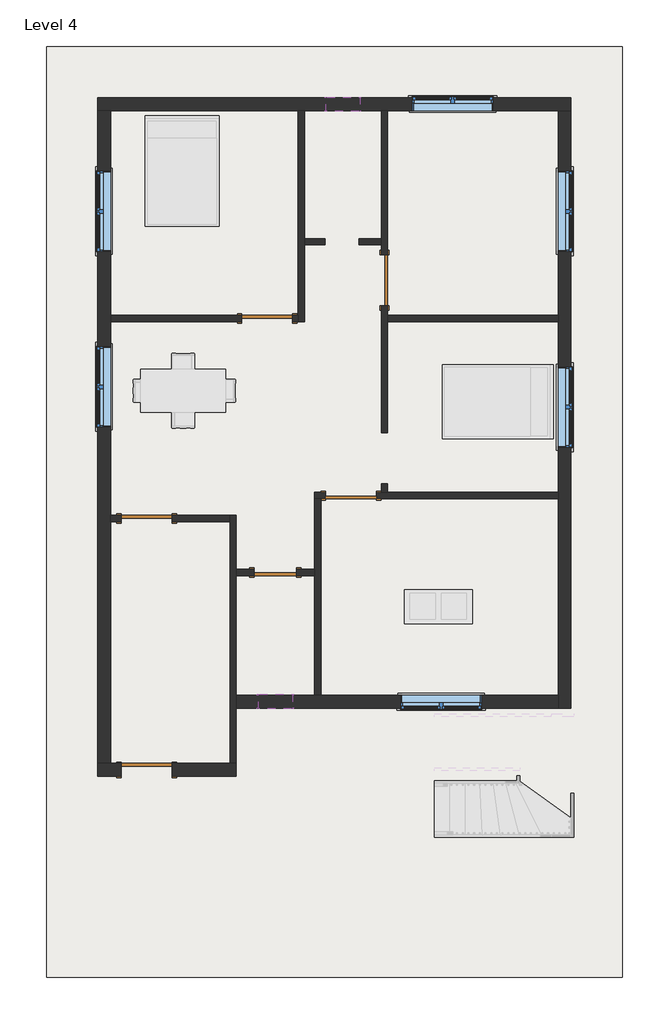
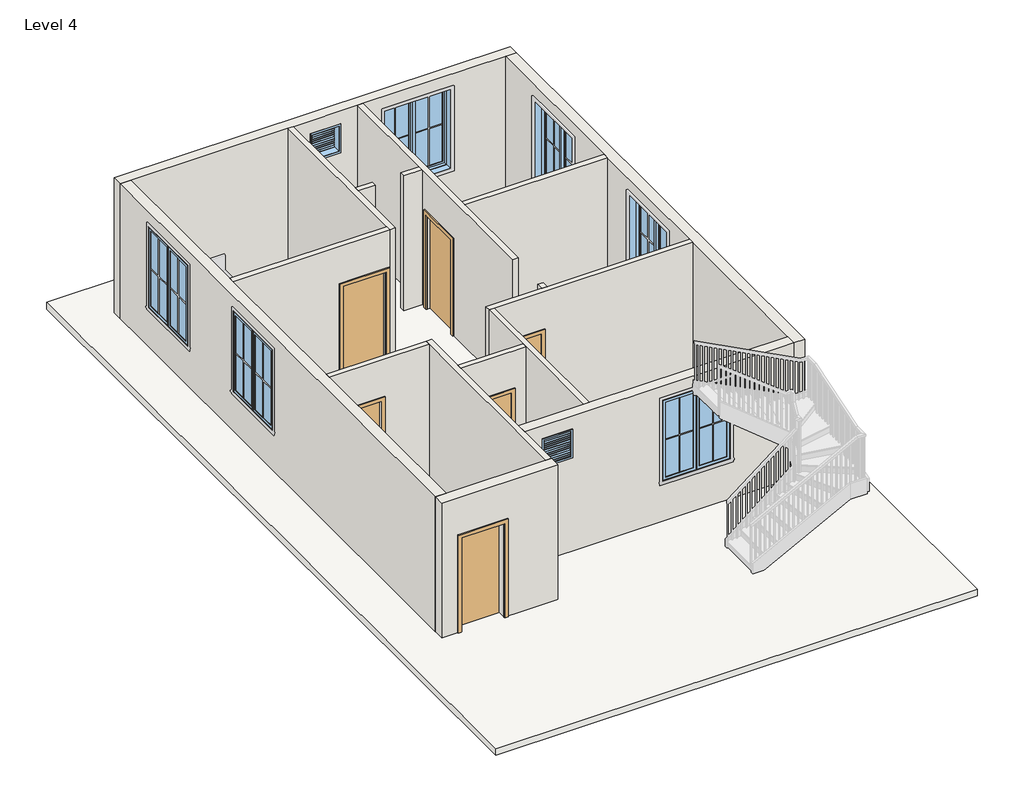
# One storey, part 1 of 3: 17 walls, 8 windows, 6 doors, 1 roof.
"""IFC4 building model written with IfcOpenShell, lengths in millimetres."""

from ifc_helpers import new_model, si_unit, frame, origin, place, context, project, spatial, polyline, outline, extrude, faceted_brep, transform, mapped, element, save
from components import door_214872d5, single_flush_door_3_e5f9f3c4, single_flush_door_3_305aa2a5, single_flush_door_3_a90ba1ad, window_9ac97e1a, window_f2d8fef0

model = new_model("IFC4")

# Units and contexts
model_context = context("Model", 3, world=origin())
ifc_project = project(units=[si_unit("LENGTHUNIT", "METRE", prefix="MILLI")], contexts=[model_context])

# Site, building, storey
site = spatial("IfcSite", under=ifc_project)
building = spatial("IfcBuilding", under=site)
storey = spatial("IfcBuildingStorey", under=building, Name="Level 4", Elevation=6400.8)

# Doors
placement = place(None, origin())
door_shape = door_214872d5(model_context)
element("IfcDoor", 1, ObjectType="Single-Flush : DOOR 2'6\"", at=placement, inside=storey, context=model_context, shape_type="MappedRepresentation", body=[
    mapped(door_shape, transform((-2309.3144966, -2885.2590409, 6400.8), x_axis=(-1.0, 0.0, 0.0), y_axis=(0.0, -1.0, 0.0), z_axis=(0.0, 0.0, 1.0))),
])
single_flush_door_3_shape = single_flush_door_3_e5f9f3c4(model_context)
element("IfcDoor", 2, ObjectType="Single-Flush : DOOR 3'", at=placement, inside=storey, context=model_context, shape_type="MappedRepresentation", body=[
    mapped(single_flush_door_3_shape, transform((-2455.3644966, 1648.6409591, 6400.8), x_axis=(1.0, 0.0, 0.0), y_axis=(0.0, 1.0, 0.0), z_axis=(0.0, 0.0, 1.0))),
])
element("IfcDoor", 3, ObjectType="Single-Flush : DOOR 3'", at=placement, inside=storey, context=model_context, shape_type="MappedRepresentation", body=[
    mapped(single_flush_door_3_shape, transform((-359.8644966, 2334.4409591, 6400.8), x_axis=(0.0, -1.0, 0.0), y_axis=(1.0, 0.0, 0.0), z_axis=(0.0, 0.0, 1.0))),
])
element("IfcDoor", 4, ObjectType="Single-Flush : DOOR 3'", at=placement, inside=storey, context=model_context, shape_type="MappedRepresentation", body=[
    mapped(single_flush_door_3_shape, transform((-956.7644966, -1513.6590409, 6400.8), x_axis=(-1.0, 0.0, 0.0), y_axis=(0.0, -1.0, 0.0), z_axis=(0.0, 0.0, 1.0))),
])
single_flush_door_3_2_shape = single_flush_door_3_305aa2a5(model_context)
element("IfcDoor", 5, ObjectType="Single-Flush : DOOR 3'", at=placement, inside=storey, context=model_context, shape_type="MappedRepresentation", body=[
    mapped(single_flush_door_3_2_shape, transform((-4608.0144966, -1920.0590409, 6400.8), x_axis=(-1.0, 0.0, 0.0), y_axis=(0.0, -1.0, 0.0), z_axis=(0.0, 0.0, 1.0))),
])
single_flush_door_3_3_shape = single_flush_door_3_a90ba1ad(model_context)
element("IfcDoor", 6, ObjectType="Single-Flush : DOOR 3'", at=placement, inside=storey, context=model_context, shape_type="MappedRepresentation", body=[
    mapped(single_flush_door_3_3_shape, transform((-4608.0144966, -6409.5090409, 6400.8), x_axis=(-1.0, 0.0, 0.0), y_axis=(0.0, -1.0, 0.0), z_axis=(0.0, 0.0, 1.0))),
])

# Roof
element("IfcRoof", 7, ObjectType="ROOF 6\"", at=placement, inside=storey, context=model_context, shape_type="SweptSolid", body=[
    extrude(outline(polyline([(-6398.7144966, 6506.3909591), (3888.2855034, 6506.3909591), (3888.2855034, -10115.6142473), (-6398.7144966, -10115.6142473), (-6398.7144966, 6506.3909591)])), frame((0.0, 0.0, 6248.4), z_axis=(0.0, 0.0, 1.0), x_axis=(1.0, 0.0, 0.0)), (0.0, 0.0, 1.0), 152.4),
])

# Walls
element("IfcWall", 8, ObjectType="WALL 4.5\"", at=placement, inside=storey, context=model_context, shape_type="Brep", body=[
    faceted_brep([(-1902.9144966, 5363.3909591, 6400.8), (-1902.9144966, 1705.7909591, 6400.8), (-1902.9144966, 1591.4909591, 6400.8), (-1902.9144966, 1591.4909591, 9448.8), (-1902.9144966, 1705.7909591, 9448.8), (-1902.9144966, 5363.3909591, 9448.8), (-1788.6144966, 5363.3909591, 6400.8), (-1788.6144966, 5363.3909591, 9448.8), (-1788.6144966, 3077.3909591, 9448.8), (-1788.6144966, 2963.0909591, 9448.8), (-1788.6144966, 1591.4909591, 9448.8), (-1788.6144966, 1591.4909591, 6400.8), (-1788.6144966, 2963.0909591, 6400.8), (-1788.6144966, 3077.3909591, 6400.8)], [[[0, 1, 2, 3, 4, 5]], [[6, 7, 8, 9, 10, 11, 12, 13]], [[2, 1, 0, 6, 13, 12, 11]], [[0, 5, 7, 6]], [[3, 2, 11, 10]], [[5, 4, 3, 10, 9, 8, 7]]]),
])
element("IfcWall", 9, ObjectType="WALL 4.5\"", at=placement, inside=storey, context=model_context, shape_type="SweptSolid", body=[
    extrude(outline(polyline([(8534.4, -1998.1644966), (6400.8, -1998.1644966), (6400.8, -1902.9144966), (9448.8, -1902.9144966), (9448.8, -5255.7144966), (6400.8, -5255.7144966), (6400.8, -2912.5644966), (8534.4, -2912.5644966), (8534.4, -1998.1644966)])), frame((0.0, 1591.4909591, 0.0), z_axis=(0.0, 1.0, 0.0), x_axis=(0.0, 0.0, 1.0)), (0.0, 0.0, 1.0), 114.3),
])
element("IfcWall", 10, ObjectType="WALL 4.5\"", at=placement, inside=storey, context=model_context, shape_type="Brep", body=[
    faceted_brep([(-417.0144966, 1877.2409591, 8534.4), (-417.0144966, 1877.2409591, 6400.8), (-417.0144966, -389.7090409, 6400.8), (-417.0144966, -389.7090409, 9448.8), (-417.0144966, 2963.0909591, 9448.8), (-417.0144966, 3077.3909591, 9448.8), (-417.0144966, 5363.3909591, 9448.8), (-417.0144966, 5363.3909591, 6400.8), (-417.0144966, 3077.3909591, 6400.8), (-417.0144966, 2963.0909591, 6400.8), (-417.0144966, 2791.6409591, 6400.8), (-417.0144966, 2791.6409591, 8534.4), (-302.7144966, -389.7090409, 6400.8), (-302.7144966, 1591.4909591, 6400.8), (-302.7144966, 1705.7909591, 6400.8), (-302.7144966, 1877.2409591, 6400.8), (-302.7144966, 1877.2409591, 8534.4), (-302.7144966, 2791.6409591, 8534.4), (-302.7144966, 2791.6409591, 6400.8), (-302.7144966, 5363.3909591, 6400.8), (-302.7144966, 5363.3909591, 9448.8), (-302.7144966, 1705.7909591, 9448.8), (-302.7144966, 1591.4909591, 9448.8), (-302.7144966, -389.7090409, 9448.8)], [[[0, 1, 2, 3, 4, 5, 6, 7, 8, 9, 10, 11]], [[12, 13, 14, 15, 16, 17, 18, 19, 20, 21, 22, 23]], [[2, 1, 15, 14, 13, 12]], [[10, 9, 8, 7, 19, 18]], [[3, 2, 12, 23]], [[7, 6, 20, 19]], [[16, 15, 1, 0]], [[17, 16, 0, 11]], [[18, 17, 11, 10]], [[6, 5, 4, 3, 23, 22, 21, 20]]]),
])
element("IfcWall", 11, ObjectType="WALL 4.5\"", at=placement, inside=storey, context=model_context, shape_type="SweptSolid", body=[
    extrude(outline(polyline([(-302.7144966, 1705.7909591), (2745.2855034, 1705.7909591), (2745.2855034, 1591.4909591), (-302.7144966, 1591.4909591), (-302.7144966, 1705.7909591)])), frame((0.0, 0.0, 6400.8), z_axis=(0.0, 0.0, 1.0), x_axis=(1.0, 0.0, 0.0)), (0.0, 0.0, 1.0), 3048.0),
])
element("IfcWall", 12, ObjectType="WALL 4.5\"", at=placement, inside=storey, context=model_context, shape_type="SweptSolid", body=[
    extrude(outline(polyline([(-1423.1234474, 2963.0909591), (-1788.6144966, 2963.0909591), (-1788.6144966, 3077.3909591), (-1423.1234474, 3077.3909591), (-1423.1234474, 2963.0909591)])), frame((0.0, 0.0, 6400.8), z_axis=(0.0, 0.0, 1.0), x_axis=(1.0, 0.0, 0.0)), (0.0, 0.0, 1.0), 3048.0),
])
element("IfcWall", 13, ObjectType="WALL 4.5\"", at=placement, inside=storey, context=model_context, shape_type="Brep", body=[
    faceted_brep([(-1413.9644966, -1456.5090409, 8534.4), (-1413.9644966, -1456.5090409, 6400.8), (-1610.8144966, -1456.5090409, 6400.8), (-1610.8144966, -1456.5090409, 9448.8), (-417.0144966, -1456.5090409, 9448.8), (-302.7144966, -1456.5090409, 9448.8), (2745.2855034, -1456.5090409, 9448.8), (2745.2855034, -1456.5090409, 6400.8), (-302.7144966, -1456.5090409, 6400.8), (-417.0144966, -1456.5090409, 6400.8), (-499.5644966, -1456.5090409, 6400.8), (-499.5644966, -1456.5090409, 8534.4), (-1610.8144966, -1570.8090409, 6400.8), (-1496.5144966, -1570.8090409, 6400.8), (-1413.9644966, -1570.8090409, 6400.8), (-1413.9644966, -1570.8090409, 8534.4), (-499.5644966, -1570.8090409, 8534.4), (-499.5644966, -1570.8090409, 6400.8), (2745.2855034, -1570.8090409, 6400.8), (2745.2855034, -1570.8090409, 9448.8), (-1496.5144966, -1570.8090409, 9448.8), (-1610.8144966, -1570.8090409, 9448.8)], [[[0, 1, 2, 3, 4, 5, 6, 7, 8, 9, 10, 11]], [[12, 13, 14, 15, 16, 17, 18, 19, 20, 21]], [[2, 1, 14, 13, 12]], [[10, 9, 8, 7, 18, 17]], [[7, 6, 19, 18]], [[3, 2, 12, 21]], [[15, 14, 1, 0]], [[16, 15, 0, 11]], [[17, 16, 11, 10]], [[6, 5, 4, 3, 21, 20, 19]]]),
])
element("IfcWall", 14, ObjectType="WALL 4.5\"", at=placement, inside=storey, context=model_context, shape_type="SweptSolid", body=[
    extrude(outline(polyline([(-302.7144966, -1304.1090409), (-302.7144966, -1456.5090409), (-417.0144966, -1456.5090409), (-417.0144966, -1304.1090409), (-302.7144966, -1304.1090409)])), frame((0.0, 0.0, 6400.8), z_axis=(0.0, 0.0, 1.0), x_axis=(1.0, 0.0, 0.0)), (0.0, 0.0, 1.0), 3048.0),
])
element("IfcWall", 15, ObjectType="WALL 4.5\"", at=placement, inside=storey, context=model_context, shape_type="Brep", body=[
    faceted_brep([(-1610.8144966, -1570.8090409, 6400.8), (-1610.8144966, -2828.1090409, 6400.8), (-1610.8144966, -2942.4090409, 6400.8), (-1610.8144966, -5076.0090409, 6400.8), (-1610.8144966, -5076.0090409, 9448.8), (-1610.8144966, -2942.4090409, 9448.8), (-1610.8144966, -2828.1090409, 9448.8), (-1610.8144966, -1570.8090409, 9448.8), (-1496.5144966, -1570.8090409, 6400.8), (-1496.5144966, -1570.8090409, 9448.8), (-1496.5144966, -5076.0090409, 9448.8), (-1496.5144966, -5076.0090409, 6400.8)], [[[0, 1, 2, 3, 4, 5, 6, 7]], [[8, 9, 10, 11]], [[3, 2, 1, 0, 8, 11]], [[0, 7, 9, 8]], [[4, 3, 11, 10]], [[7, 6, 5, 4, 10, 9]]]),
])
element("IfcWall", 16, ObjectType="WALL 4.5\"", at=placement, inside=storey, context=model_context, shape_type="SweptSolid", body=[
    extrude(outline(polyline([(6400.8, -3007.8144966), (6400.8, -2690.3144966), (8534.4, -2690.3144966), (8534.4, -1928.3144966), (6400.8, -1928.3144966), (6400.8, -1610.8144966), (9448.8, -1610.8144966), (9448.8, -3007.8144966), (6400.8, -3007.8144966)])), frame((0.0, -2942.4090409, 0.0), z_axis=(0.0, 1.0, 0.0), x_axis=(0.0, 0.0, 1.0)), (0.0, 0.0, 1.0), 114.3),
])
element("IfcWall", 17, ObjectType="WALL 4.5\"", at=placement, inside=storey, context=model_context, shape_type="Brep", body=[
    faceted_brep([(-3007.8144966, -6295.2090409, 6400.8), (-3007.8144966, -5304.6090409, 6400.8), (-3007.8144966, -5076.0090409, 6400.8), (-3007.8144966, -2942.4090409, 6400.8), (-3007.8144966, -2828.1090409, 6400.8), (-3007.8144966, -1862.9090409, 6400.8), (-3007.8144966, -1862.9090409, 9448.8), (-3007.8144966, -2828.1090409, 9448.8), (-3007.8144966, -2942.4090409, 9448.8), (-3007.8144966, -5076.0090409, 9448.8), (-3007.8144966, -5304.6090409, 9448.8), (-3007.8144966, -6295.2090409, 9448.8), (-3122.1144966, -6295.2090409, 6400.8), (-3122.1144966, -6295.2090409, 9448.8), (-3122.1144966, -1977.2090409, 9448.8), (-3122.1144966, -1862.9090409, 9448.8), (-3122.1144966, -1862.9090409, 6400.8), (-3122.1144966, -1977.2090409, 6400.8)], [[[0, 1, 2, 3, 4, 5, 6, 7, 8, 9, 10, 11]], [[12, 13, 14, 15, 16, 17]], [[5, 4, 3, 2, 1, 0, 12, 17, 16]], [[0, 11, 13, 12]], [[6, 5, 16, 15]], [[11, 10, 9, 8, 7, 6, 15, 14, 13]]]),
])
element("IfcWall", 18, ObjectType="WALL 4.5\"", at=placement, inside=storey, context=model_context, shape_type="SweptSolid", body=[
    extrude(outline(polyline([(6400.8, -5255.7144966), (6400.8, -5065.2144966), (8534.4, -5065.2144966), (8534.4, -4150.8144966), (6400.8, -4150.8144966), (6400.8, -3122.1144966), (9448.8, -3122.1144966), (9448.8, -5255.7144966), (6400.8, -5255.7144966)])), frame((0.0, -1977.2090409, 0.0), z_axis=(0.0, 1.0, 0.0), x_axis=(0.0, 0.0, 1.0)), (0.0, 0.0, 1.0), 114.3),
])
element("IfcWall", 19, ObjectType="WALL 4.5\"", at=placement, inside=storey, context=model_context, shape_type="SweptSolid", body=[
    extrude(outline(polyline([(-417.0144966, 2963.0909591), (-814.3659123, 2963.0909591), (-814.3659123, 3077.3909591), (-417.0144966, 3077.3909591), (-417.0144966, 2963.0909591)])), frame((0.0, 0.0, 6400.8), z_axis=(0.0, 0.0, 1.0), x_axis=(1.0, 0.0, 0.0)), (0.0, 0.0, 1.0), 3048.0),
])
element("IfcWall", 20, ObjectType="WALL 9\"", at=placement, inside=storey, context=model_context, shape_type="Brep", body=[
    faceted_brep([(-5484.3144966, 5363.3909591, 6400.8), (-5255.7144966, 5363.3909591, 6400.8), (-1902.9144966, 5363.3909591, 6400.8), (-1788.6144966, 5363.3909591, 6400.8), (-417.0144966, 5363.3909591, 6400.8), (-302.7144966, 5363.3909591, 6400.8), (2745.2855034, 5363.3909591, 6400.8), (2973.8855034, 5363.3909591, 6400.8), (2973.8855034, 5363.3909591, 9448.8), (2745.2855034, 5363.3909591, 9448.8), (-302.7144966, 5363.3909591, 9448.8), (-417.0144966, 5363.3909591, 9448.8), (-1788.6144966, 5363.3909591, 9448.8), (-1902.9144966, 5363.3909591, 9448.8), (-5255.7144966, 5363.3909591, 9448.8), (-5484.3144966, 5363.3909591, 9448.8), (1583.2355034, 5363.3909591, 9144.0), (1583.2355034, 5363.3909591, 7315.2), (135.4355034, 5363.3909591, 7315.2), (135.4355034, 5363.3909591, 9144.0), (-1407.6144966, 5363.3909591, 9144.0), (-798.0144966, 5363.3909591, 9144.0), (-798.0144966, 5363.3909591, 8534.4), (-1407.6144966, 5363.3909591, 8534.4), (-5484.3144966, 5591.9909591, 6400.8), (-5484.3144966, 5591.9909591, 9448.8), (2973.8855034, 5591.9909591, 9448.8), (2973.8855034, 5591.9909591, 6400.8), (1583.2355034, 5591.9909591, 9144.0), (135.4355034, 5591.9909591, 9144.0), (135.4355034, 5591.9909591, 7315.2), (1583.2355034, 5591.9909591, 7315.2), (-1407.6144966, 5591.9909591, 9144.0), (-1407.6144966, 5591.9909591, 8534.4), (-798.0144966, 5591.9909591, 8534.4), (-798.0144966, 5591.9909591, 9144.0)], [[[0, 1, 2, 3, 4, 5, 6, 7, 8, 9, 10, 11, 12, 13, 14, 15], [16, 17, 18, 19], [20, 21, 22, 23]], [[24, 25, 26, 27], [28, 29, 30, 31], [32, 33, 34, 35]], [[7, 6, 5, 4, 3, 2, 1, 0, 24, 27]], [[8, 7, 27, 26]], [[0, 15, 25, 24]], [[17, 16, 28, 31]], [[18, 17, 31, 30]], [[19, 18, 30, 29]], [[16, 19, 29, 28]], [[33, 32, 20, 23]], [[34, 33, 23, 22]], [[35, 34, 22, 21]], [[32, 35, 21, 20]], [[15, 14, 13, 12, 11, 10, 9, 8, 26, 25]]]),
])
element("IfcWall", 21, ObjectType="WALL 9\"", at=placement, inside=storey, context=model_context, shape_type="Brep", body=[
    faceted_brep([(2745.2855034, 5363.3909591, 6400.8), (2745.2855034, 1705.7909591, 6400.8), (2745.2855034, 1591.4909591, 6400.8), (2745.2855034, -1456.5090409, 6400.8), (2745.2855034, -1570.8090409, 6400.8), (2745.2855034, -5076.0090409, 6400.8), (2745.2855034, -5304.6090409, 6400.8), (2745.2855034, -5304.6090409, 9448.8), (2745.2855034, -5076.0090409, 9448.8), (2745.2855034, -1570.8090409, 9448.8), (2745.2855034, -1456.5090409, 9448.8), (2745.2855034, 1591.4909591, 9448.8), (2745.2855034, 1705.7909591, 9448.8), (2745.2855034, 5363.3909591, 9448.8), (2745.2855034, -656.4090409, 9144.0), (2745.2855034, -656.4090409, 7315.2), (2745.2855034, 791.3909591, 7315.2), (2745.2855034, 791.3909591, 9144.0), (2745.2855034, 2839.2659591, 9144.0), (2745.2855034, 2839.2659591, 7315.2), (2745.2855034, 4287.0659591, 7315.2), (2745.2855034, 4287.0659591, 9144.0), (2973.8855034, 5363.3909591, 6400.8), (2973.8855034, 5363.3909591, 9448.8), (2973.8855034, -5304.6090409, 9448.8), (2973.8855034, -5304.6090409, 6400.8), (2973.8855034, -656.4090409, 9144.0), (2973.8855034, 791.3909591, 9144.0), (2973.8855034, 791.3909591, 7315.2), (2973.8855034, -656.4090409, 7315.2), (2973.8855034, 2839.2659591, 9144.0), (2973.8855034, 4287.0659591, 9144.0), (2973.8855034, 4287.0659591, 7315.2), (2973.8855034, 2839.2659591, 7315.2)], [[[0, 1, 2, 3, 4, 5, 6, 7, 8, 9, 10, 11, 12, 13], [14, 15, 16, 17], [18, 19, 20, 21]], [[22, 23, 24, 25], [26, 27, 28, 29], [30, 31, 32, 33]], [[6, 5, 4, 3, 2, 1, 0, 22, 25]], [[0, 13, 23, 22]], [[7, 6, 25, 24]], [[15, 14, 26, 29]], [[16, 15, 29, 28]], [[17, 16, 28, 27]], [[14, 17, 27, 26]], [[19, 18, 30, 33]], [[20, 19, 33, 32]], [[21, 20, 32, 31]], [[18, 21, 31, 30]], [[13, 12, 11, 10, 9, 8, 7, 24, 23]]]),
])
element("IfcWall", 22, ObjectType="WALL 9\"", at=placement, inside=storey, context=model_context, shape_type="Brep", body=[
    faceted_brep([(2745.2855034, -5076.0090409, 6400.8), (-1496.5144966, -5076.0090409, 6400.8), (-1610.8144966, -5076.0090409, 6400.8), (-3007.8144966, -5076.0090409, 6400.8), (-3007.8144966, -5076.0090409, 9448.8), (-1610.8144966, -5076.0090409, 9448.8), (-1496.5144966, -5076.0090409, 9448.8), (2745.2855034, -5076.0090409, 9448.8), (-70.9394966, -5076.0090409, 9144.0), (-70.9394966, -5076.0090409, 7315.2), (1376.8605034, -5076.0090409, 7315.2), (1376.8605034, -5076.0090409, 9144.0), (-2004.5144966, -5076.0090409, 9144.0), (-2614.1144966, -5076.0090409, 9144.0), (-2614.1144966, -5076.0090409, 8534.4), (-2004.5144966, -5076.0090409, 8534.4), (2745.2855034, -5304.6090409, 6400.8), (2745.2855034, -5304.6090409, 9448.8), (-3007.8144966, -5304.6090409, 9448.8), (-3007.8144966, -5304.6090409, 6400.8), (-70.9394966, -5304.6090409, 9144.0), (1376.8605034, -5304.6090409, 9144.0), (1376.8605034, -5304.6090409, 7315.2), (-70.9394966, -5304.6090409, 7315.2), (-2004.5144966, -5304.6090409, 9144.0), (-2004.5144966, -5304.6090409, 8534.4), (-2614.1144966, -5304.6090409, 8534.4), (-2614.1144966, -5304.6090409, 9144.0)], [[[0, 1, 2, 3, 4, 5, 6, 7], [8, 9, 10, 11], [12, 13, 14, 15]], [[16, 17, 18, 19], [20, 21, 22, 23], [24, 25, 26, 27]], [[3, 2, 1, 0, 16, 19]], [[0, 7, 17, 16]], [[4, 3, 19, 18]], [[9, 8, 20, 23]], [[10, 9, 23, 22]], [[11, 10, 22, 21]], [[8, 11, 21, 20]], [[25, 24, 12, 15]], [[26, 25, 15, 14]], [[27, 26, 14, 13]], [[24, 27, 13, 12]], [[7, 6, 5, 4, 18, 17]]]),
])
element("IfcWall", 23, ObjectType="WALL 9\"", at=placement, inside=storey, context=model_context, shape_type="Brep", body=[
    faceted_brep([(-5065.2144966, -6295.2090409, 8534.4), (-5065.2144966, -6295.2090409, 6400.8), (-5255.7144966, -6295.2090409, 6400.8), (-5484.3144966, -6295.2090409, 6400.8), (-5484.3144966, -6295.2090409, 9448.8), (-5255.7144966, -6295.2090409, 9448.8), (-3122.1144966, -6295.2090409, 9448.8), (-3007.8144966, -6295.2090409, 9448.8), (-3007.8144966, -6295.2090409, 6400.8), (-3122.1144966, -6295.2090409, 6400.8), (-4150.8144966, -6295.2090409, 6400.8), (-4150.8144966, -6295.2090409, 8534.4), (-5484.3144966, -6523.8090409, 6400.8), (-5065.2144966, -6523.8090409, 6400.8), (-5065.2144966, -6523.8090409, 8534.4), (-4150.8144966, -6523.8090409, 8534.4), (-4150.8144966, -6523.8090409, 6400.8), (-3007.8144966, -6523.8090409, 6400.8), (-3007.8144966, -6523.8090409, 9448.8), (-5484.3144966, -6523.8090409, 9448.8)], [[[0, 1, 2, 3, 4, 5, 6, 7, 8, 9, 10, 11]], [[12, 13, 14, 15, 16, 17, 18, 19]], [[10, 9, 8, 17, 16]], [[3, 2, 1, 13, 12]], [[4, 3, 12, 19]], [[8, 7, 18, 17]], [[7, 6, 5, 4, 19, 18]], [[14, 13, 1, 0]], [[15, 14, 0, 11]], [[16, 15, 11, 10]]]),
])
element("IfcWall", 24, ObjectType="WALL 9\"", at=placement, inside=storey, context=model_context, shape_type="Brep", body=[
    faceted_brep([(-5255.7144966, -6295.2090409, 6400.8), (-5255.7144966, -1977.2090409, 6400.8), (-5255.7144966, -1862.9090409, 6400.8), (-5255.7144966, 1591.4909591, 6400.8), (-5255.7144966, 1705.7909591, 6400.8), (-5255.7144966, 5363.3909591, 6400.8), (-5255.7144966, 5363.3909591, 9448.8), (-5255.7144966, 1705.7909591, 9448.8), (-5255.7144966, 1591.4909591, 9448.8), (-5255.7144966, -1862.9090409, 9448.8), (-5255.7144966, -1977.2090409, 9448.8), (-5255.7144966, -6295.2090409, 9448.8), (-5255.7144966, 4287.0659591, 9144.0), (-5255.7144966, 4287.0659591, 7315.2), (-5255.7144966, 2839.2659591, 7315.2), (-5255.7144966, 2839.2659591, 9144.0), (-5255.7144966, 1153.3409591, 9144.0), (-5255.7144966, 1153.3409591, 7315.2), (-5255.7144966, -294.4590409, 7315.2), (-5255.7144966, -294.4590409, 9144.0), (-5484.3144966, -6295.2090409, 6400.8), (-5484.3144966, -6295.2090409, 9448.8), (-5484.3144966, 5363.3909591, 9448.8), (-5484.3144966, 5363.3909591, 6400.8), (-5484.3144966, 4287.0659591, 9144.0), (-5484.3144966, 2839.2659591, 9144.0), (-5484.3144966, 2839.2659591, 7315.2), (-5484.3144966, 4287.0659591, 7315.2), (-5484.3144966, 1153.3409591, 9144.0), (-5484.3144966, -294.4590409, 9144.0), (-5484.3144966, -294.4590409, 7315.2), (-5484.3144966, 1153.3409591, 7315.2)], [[[0, 1, 2, 3, 4, 5, 6, 7, 8, 9, 10, 11], [12, 13, 14, 15], [16, 17, 18, 19]], [[20, 21, 22, 23], [24, 25, 26, 27], [28, 29, 30, 31]], [[5, 4, 3, 2, 1, 0, 20, 23]], [[0, 11, 21, 20]], [[6, 5, 23, 22]], [[13, 12, 24, 27]], [[14, 13, 27, 26]], [[15, 14, 26, 25]], [[12, 15, 25, 24]], [[17, 16, 28, 31]], [[18, 17, 31, 30]], [[19, 18, 30, 29]], [[16, 19, 29, 28]], [[11, 10, 9, 8, 7, 6, 22, 21]]]),
])

# Windows
window_shape = window_9ac97e1a(model_context)
element("IfcWindow", 25, ObjectType="Window-Casement-Double : 57\" x 72\"", at=placement, inside=storey, context=model_context, shape_type="MappedRepresentation", body=[
    mapped(window_shape, transform((2859.5855034, 67.4909591, 6400.8), x_axis=(0.0, -1.0, 0.0), y_axis=(1.0, 0.0, 0.0), z_axis=(0.0, 0.0, 1.0))),
])
element("IfcWindow", 26, ObjectType="Window-Casement-Double : 57\" x 72\"", at=placement, inside=storey, context=model_context, shape_type="MappedRepresentation", body=[
    mapped(window_shape, transform((2859.5855034, 3563.1659591, 6400.8), x_axis=(0.0, -1.0, 0.0), y_axis=(1.0, 0.0, 0.0), z_axis=(0.0, 0.0, 1.0))),
])
element("IfcWindow", 27, ObjectType="Window-Casement-Double : 57\" x 72\"", at=placement, inside=storey, context=model_context, shape_type="MappedRepresentation", body=[
    mapped(window_shape, transform((859.3355034, 5477.6909591, 6400.8), x_axis=(1.0, 0.0, 0.0), y_axis=(0.0, 1.0, 0.0), z_axis=(0.0, 0.0, 1.0))),
])
element("IfcWindow", 28, ObjectType="Window-Casement-Double : 57\" x 72\"", at=placement, inside=storey, context=model_context, shape_type="MappedRepresentation", body=[
    mapped(window_shape, transform((-5370.0144966, 3563.1659591, 6400.8), x_axis=(0.0, 1.0, 0.0), y_axis=(-1.0, 0.0, 0.0), z_axis=(0.0, 0.0, 1.0))),
])
element("IfcWindow", 29, ObjectType="Window-Casement-Double : 57\" x 72\"", at=placement, inside=storey, context=model_context, shape_type="MappedRepresentation", body=[
    mapped(window_shape, transform((-5370.0144966, 429.4409591, 6400.8), x_axis=(0.0, 1.0, 0.0), y_axis=(-1.0, 0.0, 0.0), z_axis=(0.0, 0.0, 1.0))),
])
element("IfcWindow", 30, ObjectType="Window-Casement-Double : 57\" x 72\"", at=placement, inside=storey, context=model_context, shape_type="MappedRepresentation", body=[
    mapped(window_shape, transform((652.9605034, -5190.3090409, 6400.8), x_axis=(-1.0, 0.0, 0.0), y_axis=(0.0, -1.0, 0.0), z_axis=(0.0, 0.0, 1.0))),
])
window_2_shape = window_f2d8fef0(model_context)
element("IfcWindow", 31, ObjectType="Window-Louvers : 24\" x 24\"", at=placement, inside=storey, context=model_context, shape_type="MappedRepresentation", body=[
    mapped(window_2_shape, transform((-1102.8144966, 5484.0409591, 7620.0), x_axis=(1.0, 0.0, 0.0), y_axis=(0.0, 1.0, 0.0), z_axis=(0.0, 0.0, 1.0))),
])
element("IfcWindow", 32, ObjectType="Window-Louvers : 24\" x 24\"", at=placement, inside=storey, context=model_context, shape_type="MappedRepresentation", body=[
    mapped(window_2_shape, transform((-2309.3144966, -5196.6590409, 7620.0), x_axis=(-1.0, 0.0, 0.0), y_axis=(0.0, -1.0, 0.0), z_axis=(0.0, 0.0, 1.0))),
])

save(model, "model.ifc")

# Revit data of these elements
# Type "Single-Flush : DOOR 2'6\""
#   Type Mark = "10"
#   Construction Type Id = "MDOOR"
#   Assembly Code = "C1020"
#   Analytic Construction = "Metal"
#   Thickness = 0' - 2"
#   Heat Transfer Coefficient (U) = 0.651978 BTU/(h·ft²·°F)
#   Height = 7' - 0"
#   Trim Projection Ext = 0' - 1"
#   Trim Projection Int = 0' - 1"
#   Trim Width = 0' - 3"
#   Width = 2' - 6"
#   Define Thermal Properties by = 1
#   Door Material = Door - Panel
#   Frame Material = Door - Frame
#   Visual Light Transmittance = 0
#   Solar Heat Gain Coefficient = 0
#   Function = (empty or 0)
#   Wall Closure = (empty or 0)
# Type "Single-Flush : DOOR 3'"
#   Type Mark = "9"
#   Construction Type Id = "MDOOR"
#   Assembly Code = "C1020"
#   Analytic Construction = "Metal"
#   Thickness = 0' - 2"
#   Heat Transfer Coefficient (U) = 0.651978 BTU/(h·ft²·°F)
#   Height = 7' - 0"
#   Trim Projection Ext = 0' - 1"
#   Trim Projection Int = 0' - 1"
#   Trim Width = 0' - 3"
#   Width = 3' - 0"
#   Define Thermal Properties by = 1
#   Door Material = Door - Panel
#   Frame Material = Door - Frame
#   Visual Light Transmittance = 0
#   Solar Heat Gain Coefficient = 0
#   Function = (empty or 0)
#   Wall Closure = (empty or 0)
# Type "ROOF 6\""
#   Assembly Code = "B1020"
#   Layers, outside or top first: 0' - 6" no material (function 1)
# Type "WALL 4.5\""
#   Assembly Code = "B2010"
#   Layers, outside or top first: 0' - 4 1/2" no material (function 1)
# Type "WALL 9\""
#   Assembly Code = "B2010"
#   Layers, outside or top first: 0' - 9" no material (function 1)
# Type "Window-Casement-Double : 57\" x 72\""
#   Type Mark = "17"
#   Fire Rating = "0.5h"
#   Assembly Code = "B2020100"
#   Analytic Construction = "Double glazing - domestic"
#   Frame Extension [instance default] = 0' - 0 1/4"
#   Window Inset [instance default] = 0' - 0"
#   Wall Thickness [instance default] = 0' - 6"
#   Interior Wall Closure [instance default] = 0' - 2 1/4"
#   Half Width = 2' - 4 1/2"
#   Visual Light Transmittance = 0.81
#   Thermal Resistance (R) = 1.8146 (h·ft²·°F)/BTU
#   Solar Heat Gain Coefficient = 0.76
#   Rough Width = 4' - 9 1/2"
#   Rough Height = 6' - 0 1/2"
#   Height = 6' - 0"
#   Heat Transfer Coefficient (U) = 0.5511 BTU/(h·ft²·°F)
#   Exterior Wall Closure [instance default] = 0' - 1 1/4"
#   Extension Jamb [instance default] = 0' - 2 1/4"
#   Default Sill Height = 3' - 0"
#   Width = 4' - 9"
#   Define Thermal Properties by = 0
#   Muntin Visibility = yes
#   Interior Trim Visibility [instance default] = yes
#   Exterior Trim Visibility [instance default] = yes
#   Extension Jamb Visibility [instance default] = yes
#   Interior Trim Material = Wood - Stained
#   Muntin Pattern = Muntin Pattern_2x2 : Muntin Pattern_2x2
#   Interior Trim = Trim-Window-Interior-Flat : Picture Frame
#   Interior Frame Material = Wood - Stained
#   Glass Panel Material = Glass
#   Exterior Trim Material = Clad - White
#   Exterior Trim = Trim-Window-Exterior-Flat : with Sill
#   Exterior Frame Material = Clad - White
#   Wall Closure = (empty or 0)
# Type "Window-Louvers : 24\" x 24\""
#   Type Mark = "18"
#   Construction Type Id = "GSP4R"
#   Assembly Code = "B20"
#   Analytic Construction = "1/8 in Pilkington single glazing"
#   Visual Light Transmittance = 0.9
#   Thermal Resistance (R) = 1.53941 (h·ft²·°F)/BTU
#   Solar Heat Gain Coefficient = 0.78
#   Max Height = 1' - 11.74264"
#   Height = 2' - 0"
#   Heat Transfer Coefficient (U) = 0.6496 BTU/(h·ft²·°F)
#   Blade Width [instance default] = 1' - 10 1/2"
#   Blade Vertical Thickness = 0' - 0.35355"
#   Blade Thickness = 0' - 0 1/4"
#   Blade Spacing = 0' - 1 1/2"
#   Blade Height = 0' - 1.85355"
#   Blade Depth = 0' - 3"
#   Blade Angle = 45.00°
#   Default Sill Height = 3' - 0"
#   Trim Projection_Exterior = 0' - 0 1/2"
#   Trim Projection_Interior = 0' - 0 1/2"
#   Trim Width_Exterior = 0' - 1 1/2"
#   Trim Width_Interior = 0' - 1 1/2"
#   Width = 2' - 0"
#   Max Blade Count = 12
#   Define Thermal Properties by = 1
#   Blade Count = 12
#   Frame Material = Birch
#   Louver Material = Birch
#   Trim Exterior Material = Birch
#   Trim Interior Material = Birch
#   Wall Closure = (empty or 0)
# Element 1 (IfcDoor, "Single-Flush : DOOR 2'6\"")
#   Phase Created = New Construction
#   Materials on its faces: "Door - Frame", "Door - Panel"
# Elements 2, 3, 4, 5, 6 (IfcDoor, "Single-Flush : DOOR 3'")
#   Phase Created = New Construction
#   Materials on its faces: "Door - Frame", "Door - Panel"
# Element 7 (IfcRoof, "ROOF 6\"")
#   built-in parameter 1001705 = 21 (stored number, unit not read)
#   built-in parameter 1001701 = -0.5 (stored number, unit not read)
#   built-in parameter 1001710 = 33615
#   Phase Created = New Construction
#   Materials on its faces: "Cherry", "Default Roof", "Softwood, Lumber"
# Elements 8, 9, 10, 11, 12, 13, 14, 15, 16, 17, 18, 19 (IfcWall, "WALL 4.5\"")
#   Top Offset = 0' - 0"
#   Base Offset = 0' - 0"
#   Unconnected Height = 10' - 0"
#   wall height = 10' - 0"
#   Phase Created = New Construction
#   Base Constraint = Level 4
#   Materials on its faces: "Default Wall"
# Elements 20, 21, 22, 23, 24 (IfcWall, "WALL 9\"")
#   Top Offset = 0' - 0"
#   Base Offset = 0' - 0"
#   Unconnected Height = 10' - 0"
#   wall height = 10' - 0"
#   Phase Created = New Construction
#   Base Constraint = Level 4
#   Materials on its faces: "Default Wall"
# Element 25 (IfcWindow, "Window-Casement-Double : 57\" x 72\"")
#   Mark = "17"
#   Window Inset = 0' - 0"
#   Interior Wall Closure = 0' - 2 1/4"
#   Frame Extension = 0' - 0 1/4"
#   Exterior Wall Closure = 0' - 1 1/4"
#   Interior Trim Visibility = yes
#   Exterior Trim Visibility = yes
#   Phase Created = New Construction
#   Materials on its faces: "Wood - Stained", "Glass", "Clad - White"
# Element 26 (IfcWindow, "Window-Casement-Double : 57\" x 72\"")
#   Mark = "18"
#   Window Inset = 0' - 0"
#   Interior Wall Closure = 0' - 2 1/4"
#   Frame Extension = 0' - 0 1/4"
#   Exterior Wall Closure = 0' - 1 1/4"
#   Interior Trim Visibility = yes
#   Exterior Trim Visibility = yes
#   Phase Created = New Construction
#   Materials on its faces: "Wood - Stained", "Glass", "Clad - White"
# Element 27 (IfcWindow, "Window-Casement-Double : 57\" x 72\"")
#   Mark = "19"
#   Window Inset = 0' - 0"
#   Interior Wall Closure = 0' - 2 1/4"
#   Frame Extension = 0' - 0 1/4"
#   Exterior Wall Closure = 0' - 1 1/4"
#   Interior Trim Visibility = yes
#   Exterior Trim Visibility = yes
#   Phase Created = New Construction
#   Materials on its faces: "Wood - Stained", "Glass", "Clad - White"
# Element 28 (IfcWindow, "Window-Casement-Double : 57\" x 72\"")
#   Mark = "20"
#   Window Inset = 0' - 0"
#   Interior Wall Closure = 0' - 2 1/4"
#   Frame Extension = 0' - 0 1/4"
#   Exterior Wall Closure = 0' - 1 1/4"
#   Interior Trim Visibility = yes
#   Exterior Trim Visibility = yes
#   Phase Created = New Construction
#   Materials on its faces: "Wood - Stained", "Glass", "Clad - White"
# Element 29 (IfcWindow, "Window-Casement-Double : 57\" x 72\"")
#   Mark = "21"
#   Window Inset = 0' - 0"
#   Interior Wall Closure = 0' - 2 1/4"
#   Frame Extension = 0' - 0 1/4"
#   Exterior Wall Closure = 0' - 1 1/4"
#   Interior Trim Visibility = yes
#   Exterior Trim Visibility = yes
#   Phase Created = New Construction
#   Materials on its faces: "Wood - Stained", "Glass", "Clad - White"
# Element 30 (IfcWindow, "Window-Casement-Double : 57\" x 72\"")
#   Mark = "22"
#   Window Inset = 0' - 0"
#   Interior Wall Closure = 0' - 2 1/4"
#   Frame Extension = 0' - 0 1/4"
#   Exterior Wall Closure = 0' - 1 1/4"
#   Interior Trim Visibility = yes
#   Exterior Trim Visibility = yes
#   Phase Created = New Construction
#   Materials on its faces: "Wood - Stained", "Glass", "Clad - White"
# Element 31 (IfcWindow, "Window-Louvers : 24\" x 24\"")
#   Mark = "23"
#   Blade Width = 1' - 10 1/2"
#   Phase Created = New Construction
#   Materials on its faces: "Birch"
# Element 32 (IfcWindow, "Window-Louvers : 24\" x 24\"")
#   Mark = "24"
#   Blade Width = 1' - 10 1/2"
#   Phase Created = New Construction
#   Materials on its faces: "Birch"
# Materials
#   "Door - Panel": class "Wood", colour RGB 210 159 95, transparency 0, Cost = 0
#   "Door - Frame": colour RGB 118 70 51, transparency 0, Cost = 0
#   "Wood - Stained": class "Wood", colour RGB 224 178 126, transparency 0, Cost = 0
#   "Glass": class "Glass", colour RGB 0 128 192, transparency 0.75, Description = "Soda Lime Glass", Cost = 0
#   "Clad - White": class "Wood", colour RGB 242 242 238, transparency 0, Cost = 0
#   "Birch": class "Wood", colour RGB 224 178 126, transparency 0, Description = "Betula Alleghaniensis", Cost = 0
#   "Cherry": class "Wood", colour RGB 226 177 128, transparency 0, Description = "Prunus Serotina", Cost = 0
#   "Default Roof": colour RGB 88 101 114, transparency 0, Cost = 0
#   "Softwood, Lumber": class "Wood", colour RGB 223 192 134, transparency 0, Description = "Pinus Echinata", Cost = 0
#   "Default Wall": colour RGB 128 128 128, transparency 0, Cost = 0
